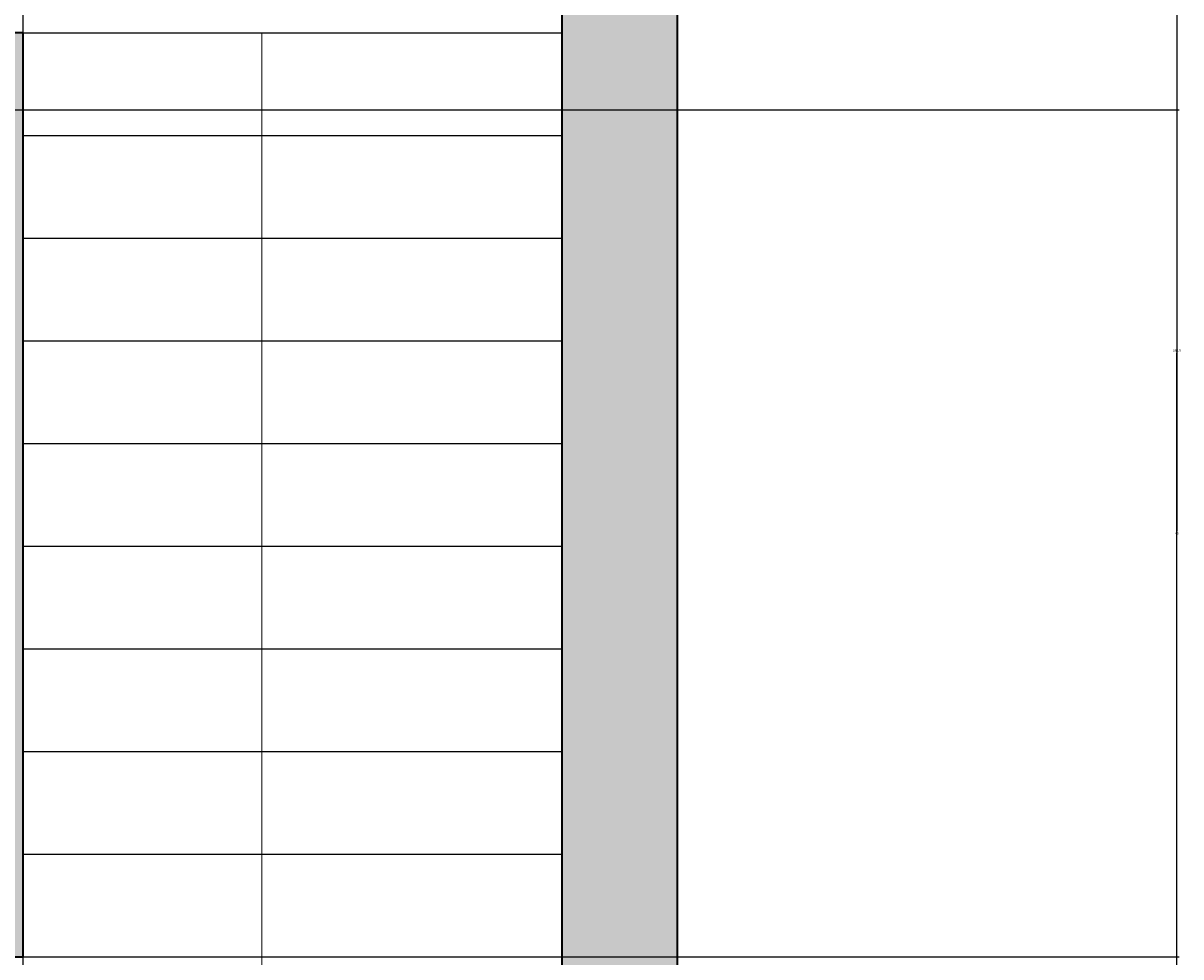
# Model space of a CAD drawing. Units: inches. Extents: x 1998 to 2588, y 1139 to 1977.
# Tile 117 of 134: x 2498 to 2588, y 1523 to 1595. Entities that reach past the tile are written whole.
import ezdxf

# ---------------------------------------------------------------- set-up
doc = ezdxf.new("R2010")
doc.units = ezdxf.units.IN
for name, color, linetype, lineweight in [('A-ANNO-DIMS', 2, 'Continuous', 18), ('A-ANNO-SYMB', 7, 'Continuous', 18), ('A-FLOR-EVTR', 7, 'Continuous', 35), ('A-FLOR-STRS', 7, 'Continuous', 25), ('A-WALL-PATT', 252, 'Continuous', 13), ('WALL', 200, 'Continuous', 35)]:
    doc.layers.add(name, color=color, linetype=linetype, lineweight=lineweight)
doc.styles.get("Standard").update_dxf_attribs({"font": 'arial.ttf'})
doc.dimstyles.get("Standard").update_dxf_attribs({"dimtxt": 0.18, "dimasz": 0.18, "dimexe": 0.18, "dimexo": 0.0625, "dimgap": 0.09, "dimtad": 0, "dimtih": 1, "dimtoh": 1, "dimdec": 4, "dimzin": 0, "dimdsep": 46, "dimtxsty": 'Standard', "dimcen": 0.09, "dimadec": 0, "dimazin": 0, "dimtfac": 1, "dimtdec": 4, "dimtofl": 0, "dimtmove": 0, "dimatfit": 3, "dimfxl": 1, "dimtolj": 1, "dimtzin": 0, "dimarcsym": 0})

# ---------------------------------------------------------------- blocks, each defined once
blk = doc.blocks.new('*D24')
at = {"layer": 'A-ANNO-DIMS', "color": 0, "lineweight": -2, "transparency": 16777216}
for p, q in [((2398.535, 1911.232), (2588.309, 1911.232)), ((2588.129, 1911.052), (2588.129, 1570.164)), ((2588.129, 1228.912), (2588.129, 1569.8)), ((2527.535, 1228.732), (2588.309, 1228.732))]:
    blk.add_line(p, q, dxfattribs=at)
at = {"layer": 'A-ANNO-DIMS', "color": 0, "transparency": 16777216}
for points in [[(2588.099, 1911.052), (2588.159, 1911.052), (2588.129, 1911.232)], [(2588.099, 1228.912), (2588.159, 1228.912), (2588.129, 1228.732)]]:
    blk.add_solid(points, dxfattribs=at)
at = {"layer": 'Defpoints', "color": 0, "transparency": 16777216}
for p in [(2398.473, 1911.232), (2588.129, 1911.232), (2527.473, 1228.732)]:
    blk.add_point(p, dxfattribs=at)
at = {"layer": 'A-ANNO-DIMS', "color": 0, "transparency": 16777216, "insert": (2588.129, 1569.982), "char_height": 0.18, "attachment_point": 5}
blk.add_mtext('\\A1;682.5', dxfattribs=at)
blk = doc.blocks.new('*D42')
at = {"layer": 'A-ANNO-DIMS', "color": 0, "lineweight": -2, "transparency": 16777216}
for p, q in [((2287.535, 1588.732), (2588.309, 1588.732)), ((2588.129, 1588.552), (2588.129, 1555.914)), ((2588.129, 1522.912), (2588.129, 1555.55)), ((2287.535, 1522.732), (2588.309, 1522.732))]:
    blk.add_line(p, q, dxfattribs=at)
at = {"layer": 'A-ANNO-DIMS', "color": 0, "transparency": 16777216}
for points in [[(2588.099, 1588.552), (2588.159, 1588.552), (2588.129, 1588.732)], [(2588.099, 1522.912), (2588.159, 1522.912), (2588.129, 1522.732)]]:
    blk.add_solid(points, dxfattribs=at)
at = {"layer": 'Defpoints', "color": 0, "transparency": 16777216}
for p in [(2287.473, 1588.732), (2588.129, 1588.732), (2287.473, 1522.732)]:
    blk.add_point(p, dxfattribs=at)
at = {"layer": 'A-ANNO-DIMS', "color": 0, "transparency": 16777216, "insert": (2588.129, 1555.732), "char_height": 0.18, "attachment_point": 5}
blk.add_mtext('\\A1;66', dxfattribs=at)

msp = doc.modelspace()

# ---------------------------------------------------------------- hatches: boundary and pattern name
at = {"layer": 'A-WALL-PATT'}
h = msp.add_hatch(color=256, dxfattribs=at)
h.dxf.hatch_style = 1
h.paths.add_polyline_path([(2527.4729, 1362.2324), (2510.9729, 1362.2324), (2510.9729, 1357.7324), (2518.4729, 1357.7324), (2518.4729, 1237.7324), (2503.1458, 1237.7324), (2503.1458, 1228.7324), (2527.4729, 1228.7324)])
h.paths.add_polyline_path([(2490.5682, 1362.2324), (2398.4729, 1362.2324), (2398.4729, 1357.7324), (2490.5682, 1357.7324)])
h.paths.add_polyline_path([(2224.9729, 1264.7324), (2222.9729, 1264.7324), (2222.9729, 1232.4125), (2341.4729, 1232.4125), (2341.4729, 1234.4125), (2224.9729, 1234.4125)])
h.paths.add_polyline_path([(2334.5332, 1273.7324), (2264.7638, 1273.7324), (2264.7638, 1269.5611, -0.043659), (2264.3413, 1264.7324), (2334.5332, 1264.7324)])
h.paths.add_polyline_path([(2236.9551, 1273.7324), (2234.4125, 1273.7324), (2234.4125, 1264.7324), (2236.9551, 1264.7324), (2236.9551, 1269.5611)])
h.paths.add_polyline_path([(2222.9729, 1293.2324), (2096.9729, 1293.2324), (2096.9729, 1345.0966), (2087.9729, 1345.0966), (2087.9729, 1284.2324), (2222.9729, 1284.2324), (2222.9729, 1285.137)])
h.paths.add_polyline_path([(2096.9729, 1458.7927), (2087.9729, 1458.7927), (2087.9729, 1417.7324), (2087.9729, 1413.2324), (2096.9729, 1413.2324), (2096.9729, 1417.7324)])
h.paths.add_polyline_path([(2096.9729, 1413.2324), (2087.9729, 1413.2324), (2087.9729, 1365.5012), (2096.9729, 1365.5012), (2096.9729, 1369.3358)])
h.paths.add_polyline_path([(2186.2943, 1417.7324), (2138.6074, 1417.7324), (2096.9729, 1417.7324), (2096.9729, 1413.2324), (2138.6074, 1413.2324), (2186.2943, 1413.2324)])
h.paths.add_polyline_path([(2181.4729, 1465.7324), (2176.9729, 1465.7324), (2176.9729, 1451.6434), (2181.4729, 1451.6434)])
h.paths.add_polyline_path([(2181.4729, 1422.1664), (2176.9729, 1422.1664), (2176.9729, 1417.7324), (2181.4729, 1417.7324)])
h.paths.add_polyline_path([(2063.9729, 1465.7324), (2087.9729, 1465.7324), (2087.9729, 1470.2324), (2059.4729, 1470.2324), (2059.4729, 1413.2324), (2087.9729, 1413.2324), (2087.9729, 1417.7324), (2063.9729, 1417.7324)])
h.paths.add_polyline_path([(2181.4729, 1755.2324), (2176.9729, 1755.2324), (2176.9729, 1748.6798), (2177.0513, 1748.6798), (2181.4729, 1748.6798)])
h.paths.add_polyline_path([(2227.4729, 1707.2324), (2220.4647, 1707.2324), (2220.4647, 1702.7324), (2222.9729, 1702.7324), (2222.9729, 1604.637), (2227.4729, 1604.637)])
h.paths.add_polyline_path([(2114.9729, 1702.7324), (2105.9729, 1702.7324), (2105.9729, 1628.4781, -0.0318759), (2110.1012, 1628.7416), (2114.9729, 1628.7416)])
h.paths.add_polyline_path([(2345.9729, 1739.3278), (2341.4729, 1739.3278), (2341.4729, 1647.5211), (2345.9729, 1647.5211)])
h.paths.add_polyline_path([(2350.6273, 1641.2324), (2345.9729, 1641.2324), (2345.9729, 1636.7324), (2350.6273, 1636.7324), (2350.6273, 1639.8729)])
h.paths.add_polyline_path([(2501.9729, 1641.2324), (2407.9729, 1641.2324), (2392.5005, 1641.2324), (2392.5005, 1639.8729), (2392.5005, 1636.7324), (2501.9729, 1636.7324)])
h.paths.add_polyline_path([(2510.9729, 1755.2324), (2501.9729, 1755.2324), (2501.9729, 1641.2324), (2510.9729, 1641.2324)])
h.paths.add_polyline_path([(2549.1786, 1641.2324), (2522.3775, 1641.2324), (2522.3775, 1636.7324), (2540.1786, 1636.7324), (2540.1786, 1480.7324), (2522.3775, 1480.7324), (2522.3775, 1476.2324), (2549.1786, 1476.2324)])
h.paths.add_polyline_path([(2498.1786, 1594.7324), (2407.9729, 1594.7324), (2407.9729, 1585.7324), (2416.9729, 1585.7324), (2489.1786, 1585.7324), (2489.1786, 1531.7324), (2416.9729, 1531.7324), (2407.9729, 1531.7324), (2407.9729, 1522.7324), (2498.1786, 1522.7324)])
h.paths.add_polyline_path([(2351.6437, 1480.7324), (2345.9729, 1480.7324), (2345.9729, 1476.2324), (2351.6437, 1476.2324), (2351.6437, 1477.5919)])
h.paths.add_polyline_path([(2501.9729, 1480.7324), (2498.1786, 1480.7324), (2407.9729, 1480.7324), (2393.5168, 1480.7324), (2393.5168, 1477.5919), (2393.5168, 1476.2324), (2501.9729, 1476.2324)])

# ---------------------------------------------------------------- linework, layer by layer
at = {"layer": 'A-ANNO-SYMB'}
msp.add_line((2516.7914, 1594.7324), (2516.7914, 1507.2016), dxfattribs=at)
at = {"layer": 'A-FLOR-EVTR'}
msp.add_lwpolyline([(2407.9729, 1522.7324), (2498.1786, 1522.7324), (2498.1786, 1594.7324), (2407.9729, 1594.7324)], close=True, dxfattribs=at)
at = {"layer": 'A-FLOR-STRS'}
for p, q in [((2498.1786, 1480.7324), (2498.1786, 1636.7324)), ((2407.9729, 1594.7324), (2540.1786, 1594.7324)), ((2498.1786, 1586.7324), (2540.1786, 1586.7324)), ((2498.1786, 1578.7324), (2540.1786, 1578.7324)), ((2498.1786, 1570.7324), (2540.1786, 1570.7324)), ((2498.1786, 1562.7324), (2540.1786, 1562.7324)), ((2498.1786, 1554.7324), (2540.1786, 1554.7324)), ((2498.1786, 1546.7324), (2540.1786, 1546.7324)), ((2498.1786, 1538.7324), (2540.1786, 1538.7324)), ((2498.1786, 1530.7324), (2540.1786, 1530.7324))]:
    msp.add_line(p, q, dxfattribs=at)
at = {"layer": 'WALL'}
for p, q in [((2549.1786, 1641.2324), (2549.1786, 1476.2324)), ((2540.1786, 1636.7324), (2540.1786, 1480.7324))]:
    msp.add_line(p, q, dxfattribs=at)

# ---------------------------------------------------------------- dimensions: what is measured, and where the dimension line sits
at = {"layer": 'A-ANNO-DIMS'}
for base, p1, p2, override, picture, middle in [((2588.1286, 1911.2324), (2527.4729, 1228.7324), (2398.4729, 1911.2324), {"dimdec": 1, "dimlfac": 1, "dimrnd": 0, "dimzin": 0, "dimdsep": 46, "dimlunit": 2}, '*D24', (2588.1286, 1569.9824)), ((2588.1286, 1588.7324), (2287.4729, 1522.7324), (2287.4729, 1588.7324), {"dimdec": 0, "dimlfac": 1, "dimrnd": 0, "dimzin": 0, "dimdsep": 46, "dimlunit": 2}, '*D42', (2588.1286, 1555.7324))]:
    dim = msp.add_linear_dim(base=base, p1=p1, p2=p2, angle=90, dimstyle='Standard', override=override, dxfattribs=at)
    dim.commit()
    dim.dimension.update_dxf_attribs({"geometry": picture, "text_midpoint": middle})

doc.saveas('drawing.dxf')
